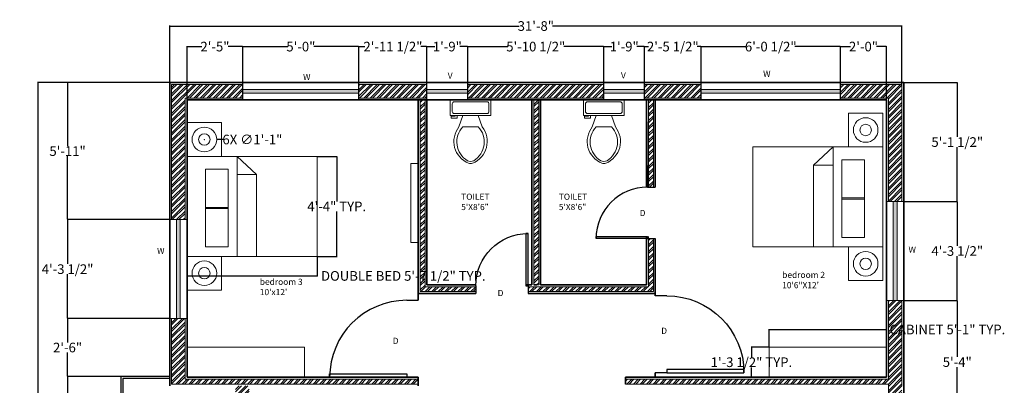
# Model space of a CAD drawing. Units: inches. Extents: x -340 to 394, y 381 to 1380.
# Tile 3 of 3: x -117 to 394, y 757 to 947. Entities that reach past the tile are written whole.
import ezdxf

# ---------------------------------------------------------------- set-up
doc = ezdxf.new("R2010")
doc.units = ezdxf.units.IN
doc.header["$MEASUREMENT"] = 0
for name, color, linetype, lineweight in [('A-ANNO-DIMS', 150, 'Continuous', 18), ('A-ANNO-TEXT', 11, 'Continuous', 18), ('A-AREA-IDEN', 11, 'Continuous', 18), ('A-FLOR', 150, 'Continuous', 25), ('A-FLOR-CASE', 130, 'Continuous', 20), ('A-FLOR-FIXT', 130, 'Continuous', 18), ('A-GLAZ-PATT', 220, 'Continuous', 13), ('A-WALL-FNSH', 150, 'Continuous', 18), ('A-WALL-PATT', 10, 'Continuous', 13), ('door', 200, 'Continuous', 25), ('fur', 130, 'Continuous', 18), ('wall', 150, 'Continuous', 35), ('wind', 220, 'Continuous', 20)]:
    doc.layers.add(name, color=color, linetype=linetype, lineweight=lineweight)
doc.styles.get("Standard").update_dxf_attribs({"font": 'arial.ttf'})
doc.dimstyles.get("Standard").update_dxf_attribs({"dimtxt": 5, "dimasz": 0.18, "dimexe": 0.18, "dimexo": 0.0625, "dimgap": 0.09, "dimtad": 0, "dimtih": 1, "dimtoh": 1, "dimdec": 0, "dimzin": 0, "dimdsep": 46, "dimlunit": 4, "dimtxsty": 'Standard', "dimcen": 0.09, "dimadec": 0, "dimazin": 0, "dimtfac": 1, "dimtdec": 0, "dimtofl": 0, "dimtmove": 0, "dimatfit": 3, "dimfxl": 1, "dimtolj": 1, "dimtzin": 0, "dimarcsym": 0})

# ---------------------------------------------------------------- blocks, each defined once
blk = doc.blocks.new('*U2')
for p, q in [((0, 0), (0, -6)), ((40, 0), (40, -6))]:
    blk.add_line(p, q)
blk.add_lwpolyline([(0, 0), (0, 40), (1.75, 40), (1.75, 0)], close=True)
blk.add_arc((0, 0), 40, 0, 90)
blk = doc.blocks.new('*U4')
for p, q in [((9.5, -6), (9.5, -2)), ((-10, -8.5), (-8, -8.5)), ((-10, -9.5), (-10, -8.5)), ((-7, -9.5), (-10, -9.5)), ((-8, -8.5), (-8, -8)), ((-7, -8), (-7, -9.5)), ((-4, -8), (-6, -14)), ((4, -8), (6, -14)), ((4, -14), (-4, -14))]:
    blk.add_line(p, q)
blk.add_lwpolyline([(10.5, -8), (10.5, 0), (-10.5, 0), (-10.5, -8)], close=True)
for points in [[(-9.5, -2), (-9.5, -6)], [(8.5, -1), (-8.5, -1)], [(-8.5, -7), (8.5, -7)]]:
    blk.add_lwpolyline(points)
for centre, radius, start, end in [((-8.62, -1.88), 0.884, 81.8699, 188.1301), ((8.62, -1.88), 0.884, 351.8699, 98.1301), ((-8.62, -6.12), 0.884, 171.8699, 278.1301), ((8.62, -6.12), 0.884, 261.8699, 8.1301), ((3.52, -21.58), 12.17, 141.4691, 247.9714), ((4.2, -21.82), 11.33, 136.3677, 238.9468), ((-3.52, -21.58), 12.17, 292.0284, 38.5307), ((-4.2, -21.82), 11.33, 301.053, 43.6321), ((0, -27.88), 4, 245.7318, 294.2682), ((0, -29), 4, 254.8605, 285.1395)]:
    blk.add_arc(centre, radius, start, end)
blk = doc.blocks.new('*D5')
at = {"layer": 'A-ANNO-DIMS', "color": 0, "lineweight": -2, "transparency": 16777216}
for p, q in [((-39.62, 914.26), (-39.62, 943.76)), ((-39.44, 943.58), (141.71, 943.58)), ((340.2, 943.58), (159.06, 943.58)), ((340.38, 913.26), (340.38, 943.76))]:
    blk.add_line(p, q, dxfattribs=at)
at = {"layer": 'A-ANNO-DIMS', "color": 0, "transparency": 16777216}
for points in [[(-39.44, 943.61), (-39.44, 943.55), (-39.62, 943.58)], [(340.2, 943.61), (340.2, 943.55), (340.38, 943.58)]]:
    blk.add_solid(points, dxfattribs=at)
at = {"layer": 'Defpoints', "color": 0, "transparency": 16777216}
for p in [(340.38, 943.58), (-39.62, 914.2), (340.38, 913.2)]:
    blk.add_point(p, dxfattribs=at)
at = {"layer": 'A-ANNO-DIMS', "color": 0, "transparency": 16777216, "insert": (150.38, 943.58), "char_height": 5, "attachment_point": 5}
blk.add_mtext('\\A1;31\'-8"', dxfattribs=at)
blk = doc.blocks.new('*D6')
at = {"layer": 'A-ANNO-DIMS', "color": 0, "lineweight": -2, "transparency": 16777216}
for p, q in [((-39.68, 914.2), (-108.24, 914.2)), ((-108.06, 914.02), (-108.06, 693.34)), ((-108.06, 467.38), (-108.06, 688.05)), ((-39.68, 467.2), (-108.24, 467.2))]:
    blk.add_line(p, q, dxfattribs=at)
at = {"layer": 'A-ANNO-DIMS', "color": 0, "transparency": 16777216}
for points in [[(-108.09, 914.02), (-108.03, 914.02), (-108.06, 914.2)], [(-108.09, 467.38), (-108.03, 467.38), (-108.06, 467.2)]]:
    blk.add_solid(points, dxfattribs=at)
at = {"layer": 'Defpoints', "color": 0, "transparency": 16777216}
for p in [(-39.62, 914.2), (-108.06, 467.2), (-39.62, 467.2)]:
    blk.add_point(p, dxfattribs=at)
at = {"layer": 'A-ANNO-DIMS', "color": 0, "transparency": 16777216, "insert": (-108.06, 690.7), "char_height": 5, "attachment_point": 5}
blk.add_mtext('\\A1;37\'-3"', dxfattribs=at)
blk = doc.blocks.new('BED-DOUBLE')
for p, q in [((25.93, 0), (25.93, 51.94)), ((25.93, 51.94), (25.93, 42.46)), ((36.06, 42.46), (25.93, 51.94)), ((25.93, 51.94), (36.06, 42.46)), ((25.93, 42.46), (36.06, 42.46)), ((36.06, 42.46), (36.06, 0))]:
    blk.add_line(p, q)
for points in [[(0, 0), (67.52, 0), (67.52, 51.94), (0, 51.94)], [(9.57, 24.81), (21.34, 24.81), (21.34, 45.28), (9.57, 45.28)], [(9.57, 4.93), (21.34, 4.93), (21.34, 25.4), (9.57, 25.4)]]:
    blk.add_lwpolyline(points, close=True)
blk = doc.blocks.new('NIGHTSTAND')
blk.add_lwpolyline([(0, 0), (17.94, 0), (17.94, 17.5), (0, 17.5)], close=True)
for radius in [6.39, 2.96]:
    blk.add_circle((8.97, 8.75), radius)
blk = doc.blocks.new('CABINET-BEDROOM')
blk.add_lwpolyline([(0, 0), (60.98, 0), (60.98, 15.69), (0, 15.69)], close=True)
blk = doc.blocks.new('*D15')
at = {"layer": 'A-ANNO-DIMS', "color": 0, "lineweight": -2, "transparency": 16777216}
for p, q in [((-30.62, 823.92), (-30.62, 813.67)), ((36.9, 823.92), (36.9, 813.67)), ((-30.44, 813.85), (36.72, 813.85)), ((36.9, 813.85), (37.08, 813.85))]:
    blk.add_line(p, q, dxfattribs=at)
at = {"layer": 'A-ANNO-DIMS', "color": 0, "transparency": 16777216}
for points in [[(-30.44, 813.88), (-30.44, 813.82), (-30.62, 813.85)], [(36.72, 813.88), (36.72, 813.82), (36.9, 813.85)]]:
    blk.add_solid(points, dxfattribs=at)
at = {"layer": 'Defpoints', "color": 0, "transparency": 16777216}
for p in [(-30.62, 823.98), (36.9, 823.98), (36.9, 813.85)]:
    blk.add_point(p, dxfattribs=at)
at = {"layer": 'A-ANNO-DIMS', "color": 0, "transparency": 16777216, "insert": (81.59, 813.85), "char_height": 5, "attachment_point": 5}
blk.add_mtext('\\A1;DOUBLE BED 5\'-7 1/2" TYP.', dxfattribs=at)
blk = doc.blocks.new('*D16')
at = {"layer": 'A-ANNO-DIMS', "color": 0, "lineweight": -2, "transparency": 16777216}
for p, q in [((36.96, 875.92), (47.21, 875.92)), ((47.03, 875.74), (47.03, 852.54)), ((47.03, 824.16), (47.03, 847.36)), ((36.96, 823.98), (47.21, 823.98))]:
    blk.add_line(p, q, dxfattribs=at)
at = {"layer": 'A-ANNO-DIMS', "color": 0, "transparency": 16777216}
for points in [[(47, 875.74), (47.06, 875.74), (47.03, 875.92)], [(47, 824.16), (47.06, 824.16), (47.03, 823.98)]]:
    blk.add_solid(points, dxfattribs=at)
at = {"layer": 'Defpoints', "color": 0, "transparency": 16777216}
for p in [(36.9, 875.92), (47.03, 875.92), (36.9, 823.98)]:
    blk.add_point(p, dxfattribs=at)
at = {"layer": 'A-ANNO-DIMS', "color": 0, "transparency": 16777216, "insert": (47.03, 849.95), "char_height": 5, "attachment_point": 5}
blk.add_mtext('\\A1;4\'-4" TYP.', dxfattribs=at)
blk = doc.blocks.new('*D17')
at = {"layer": 'A-ANNO-DIMS', "color": 0, "lineweight": -2, "transparency": 16777216}
for p, q in [((271.4, 776.95), (271.4, 786.21)), ((271.58, 786.03), (332.2, 786.03)), ((332.38, 776.95), (332.38, 786.21)), ((332.38, 786.03), (332.56, 786.03))]:
    blk.add_line(p, q, dxfattribs=at)
at = {"layer": 'A-ANNO-DIMS', "color": 0, "transparency": 16777216}
for points in [[(271.58, 786.06), (271.58, 786), (271.4, 786.03)], [(332.2, 786.06), (332.2, 786), (332.38, 786.03)]]:
    blk.add_solid(points, dxfattribs=at)
at = {"layer": 'Defpoints', "color": 0, "transparency": 16777216}
for p in [(332.38, 786.03), (271.4, 776.89), (332.38, 776.89)]:
    blk.add_point(p, dxfattribs=at)
at = {"layer": 'A-ANNO-DIMS', "color": 0, "transparency": 16777216, "insert": (363.97, 786.03), "char_height": 5, "attachment_point": 5}
blk.add_mtext('\\A1;CABINET 5\'-1" TYP.', dxfattribs=at)
blk = doc.blocks.new('*D18')
at = {"layer": 'A-ANNO-DIMS', "color": 0, "lineweight": -2, "transparency": 16777216}
for p, q in [((271.34, 776.89), (262.08, 776.89)), ((262.26, 776.71), (262.26, 771.72)), ((262.26, 761.38), (262.26, 766.37)), ((271.34, 761.2), (262.08, 761.2))]:
    blk.add_line(p, q, dxfattribs=at)
at = {"layer": 'A-ANNO-DIMS', "color": 0, "transparency": 16777216}
for points in [[(262.23, 776.71), (262.29, 776.71), (262.26, 776.89)], [(262.23, 761.38), (262.29, 761.38), (262.26, 761.2)]]:
    blk.add_solid(points, dxfattribs=at)
at = {"layer": 'Defpoints', "color": 0, "transparency": 16777216}
for p in [(262.26, 776.89), (271.4, 776.89), (271.4, 761.2)]:
    blk.add_point(p, dxfattribs=at)
at = {"layer": 'A-ANNO-DIMS', "color": 0, "transparency": 16777216, "insert": (262.26, 769.04), "char_height": 5, "attachment_point": 5}
blk.add_mtext('\\A1;1\'-3 1/2" TYP.', dxfattribs=at)
blk = doc.blocks.new('*D29')
at = {"layer": 'A-ANNO-DIMS', "color": 0, "lineweight": -2, "transparency": 16777216}
for p, q in [((341.44, 801.11), (369.26, 801.11)), ((369.08, 800.93), (369.08, 771.76)), ((369.08, 737.33), (369.08, 766.49)), ((341.44, 737.15), (369.26, 737.15))]:
    blk.add_line(p, q, dxfattribs=at)
at = {"layer": 'A-ANNO-DIMS', "color": 0, "transparency": 16777216}
for points in [[(369.05, 800.93), (369.11, 800.93), (369.08, 801.11)], [(369.05, 737.33), (369.11, 737.33), (369.08, 737.15)]]:
    blk.add_solid(points, dxfattribs=at)
at = {"layer": 'Defpoints', "color": 0, "transparency": 16777216}
for p in [(341.38, 801.11), (369.08, 801.11), (341.38, 737.15)]:
    blk.add_point(p, dxfattribs=at)
at = {"layer": 'A-ANNO-DIMS', "color": 0, "transparency": 16777216, "insert": (369.08, 769.13), "char_height": 5, "attachment_point": 5}
blk.add_mtext('\\A1;5\'-4"', dxfattribs=at)
blk = doc.blocks.new('*D30')
at = {"layer": 'A-ANNO-DIMS', "color": 0, "lineweight": -2, "transparency": 16777216}
for p, q in [((341.44, 852.47), (369.26, 852.47)), ((369.08, 852.29), (369.08, 829.47)), ((369.08, 801.29), (369.08, 824.11)), ((341.44, 801.11), (369.26, 801.11))]:
    blk.add_line(p, q, dxfattribs=at)
at = {"layer": 'A-ANNO-DIMS', "color": 0, "transparency": 16777216}
for points in [[(369.05, 852.29), (369.11, 852.29), (369.08, 852.47)], [(369.05, 801.29), (369.11, 801.29), (369.08, 801.11)]]:
    blk.add_solid(points, dxfattribs=at)
at = {"layer": 'Defpoints', "color": 0, "transparency": 16777216}
for p in [(341.38, 852.47), (369.08, 852.47), (341.38, 801.11)]:
    blk.add_point(p, dxfattribs=at)
at = {"layer": 'A-ANNO-DIMS', "color": 0, "transparency": 16777216, "insert": (369.08, 826.79), "char_height": 5, "attachment_point": 5}
blk.add_mtext('\\A1;4\'-3 1/2"', dxfattribs=at)
blk = doc.blocks.new('*D31')
at = {"layer": 'A-ANNO-DIMS', "color": 0, "lineweight": -2, "transparency": 16777216}
for p, q in [((341.44, 914.2), (369.26, 914.2)), ((369.08, 914.02), (369.08, 886.01)), ((369.08, 852.65), (369.08, 880.66)), ((341.44, 852.47), (369.26, 852.47))]:
    blk.add_line(p, q, dxfattribs=at)
at = {"layer": 'A-ANNO-DIMS', "color": 0, "transparency": 16777216}
for points in [[(369.05, 914.02), (369.11, 914.02), (369.08, 914.2)], [(369.05, 852.65), (369.11, 852.65), (369.08, 852.47)]]:
    blk.add_solid(points, dxfattribs=at)
at = {"layer": 'Defpoints', "color": 0, "transparency": 16777216}
for p in [(341.38, 914.2), (369.08, 914.2), (341.38, 852.47)]:
    blk.add_point(p, dxfattribs=at)
at = {"layer": 'A-ANNO-DIMS', "color": 0, "transparency": 16777216, "insert": (369.08, 883.34), "char_height": 5, "attachment_point": 5}
blk.add_mtext('\\A1;5\'-1 1/2"', dxfattribs=at)
blk = doc.blocks.new('*D32')
at = {"layer": 'A-ANNO-DIMS', "color": 0, "lineweight": -2, "transparency": 16777216}
for p, q in [((-30.62, 905.26), (-30.62, 933.08)), ((-30.44, 932.9), (-22.93, 932.9)), ((-1.86, 932.9), (-9.37, 932.9)), ((-1.68, 905.26), (-1.68, 933.08))]:
    blk.add_line(p, q, dxfattribs=at)
at = {"layer": 'A-ANNO-DIMS', "color": 0, "transparency": 16777216}
for points in [[(-30.44, 932.93), (-30.44, 932.87), (-30.62, 932.9)], [(-1.86, 932.93), (-1.86, 932.87), (-1.68, 932.9)]]:
    blk.add_solid(points, dxfattribs=at)
at = {"layer": 'Defpoints', "color": 0, "transparency": 16777216}
for p in [(-1.68, 932.9), (-30.62, 905.2), (-1.68, 905.2)]:
    blk.add_point(p, dxfattribs=at)
at = {"layer": 'A-ANNO-DIMS', "color": 0, "transparency": 16777216, "insert": (-16.15, 932.9), "char_height": 5, "attachment_point": 5}
blk.add_mtext('\\A1;2\'-5"', dxfattribs=at)
blk = doc.blocks.new('*D33')
at = {"layer": 'A-ANNO-DIMS', "color": 0, "lineweight": -2, "transparency": 16777216}
for p, q in [((-1.68, 905.26), (-1.68, 933.08)), ((-1.5, 932.9), (21.71, 932.9)), ((58.38, 932.9), (35.18, 932.9)), ((58.56, 905.26), (58.56, 933.08))]:
    blk.add_line(p, q, dxfattribs=at)
at = {"layer": 'A-ANNO-DIMS', "color": 0, "transparency": 16777216}
for points in [[(-1.5, 932.93), (-1.5, 932.87), (-1.68, 932.9)], [(58.38, 932.93), (58.38, 932.87), (58.56, 932.9)]]:
    blk.add_solid(points, dxfattribs=at)
at = {"layer": 'Defpoints', "color": 0, "transparency": 16777216}
for p in [(58.56, 932.9), (-1.68, 905.2), (58.56, 905.2)]:
    blk.add_point(p, dxfattribs=at)
at = {"layer": 'A-ANNO-DIMS', "color": 0, "transparency": 16777216, "insert": (28.44, 932.9), "char_height": 5, "attachment_point": 5}
blk.add_mtext('\\A1;5\'-0"', dxfattribs=at)
blk = doc.blocks.new('*D34')
at = {"layer": 'A-ANNO-DIMS', "color": 0, "lineweight": -2, "transparency": 16777216}
for p, q in [((58.56, 905.26), (58.56, 933.08)), ((58.74, 932.9), (61.68, 932.9)), ((93.7, 932.9), (90.77, 932.9)), ((93.88, 905.26), (93.88, 933.08))]:
    blk.add_line(p, q, dxfattribs=at)
at = {"layer": 'A-ANNO-DIMS', "color": 0, "transparency": 16777216}
for points in [[(58.74, 932.93), (58.74, 932.87), (58.56, 932.9)], [(93.7, 932.93), (93.7, 932.87), (93.88, 932.9)]]:
    blk.add_solid(points, dxfattribs=at)
at = {"layer": 'Defpoints', "color": 0, "transparency": 16777216}
for p in [(93.88, 932.9), (58.56, 905.2), (93.88, 905.2)]:
    blk.add_point(p, dxfattribs=at)
at = {"layer": 'A-ANNO-DIMS', "color": 0, "transparency": 16777216, "insert": (76.22, 932.9), "char_height": 5, "attachment_point": 5}
blk.add_mtext('\\A1;2\'-11 1/2"', dxfattribs=at)
blk = doc.blocks.new('*D35')
at = {"layer": 'A-ANNO-DIMS', "color": 0, "lineweight": -2, "transparency": 16777216}
for p, q in [((93.88, 905.26), (93.88, 933.08)), ((94.06, 932.9), (97.95, 932.9)), ((114.84, 932.9), (110.95, 932.9)), ((115.02, 905.26), (115.02, 933.08))]:
    blk.add_line(p, q, dxfattribs=at)
at = {"layer": 'A-ANNO-DIMS', "color": 0, "transparency": 16777216}
for points in [[(94.06, 932.93), (94.06, 932.87), (93.88, 932.9)], [(114.84, 932.93), (114.84, 932.87), (115.02, 932.9)]]:
    blk.add_solid(points, dxfattribs=at)
at = {"layer": 'Defpoints', "color": 0, "transparency": 16777216}
for p in [(115.02, 932.9), (93.88, 905.2), (115.02, 905.2)]:
    blk.add_point(p, dxfattribs=at)
at = {"layer": 'A-ANNO-DIMS', "color": 0, "transparency": 16777216, "insert": (104.45, 932.9), "char_height": 5, "attachment_point": 5}
blk.add_mtext('\\A1;1\'-9"', dxfattribs=at)
blk = doc.blocks.new('*D36')
at = {"layer": 'A-ANNO-DIMS', "color": 0, "lineweight": -2, "transparency": 16777216}
for p, q in [((115.02, 905.26), (115.02, 933.08)), ((115.2, 932.9), (135.84, 932.9)), ((185.49, 932.9), (164.85, 932.9)), ((185.67, 905.26), (185.67, 933.08))]:
    blk.add_line(p, q, dxfattribs=at)
at = {"layer": 'A-ANNO-DIMS', "color": 0, "transparency": 16777216}
for points in [[(115.2, 932.93), (115.2, 932.87), (115.02, 932.9)], [(185.49, 932.93), (185.49, 932.87), (185.67, 932.9)]]:
    blk.add_solid(points, dxfattribs=at)
at = {"layer": 'Defpoints', "color": 0, "transparency": 16777216}
for p in [(185.67, 932.9), (115.02, 905.2), (185.67, 905.2)]:
    blk.add_point(p, dxfattribs=at)
at = {"layer": 'A-ANNO-DIMS', "color": 0, "transparency": 16777216, "insert": (150.34, 932.9), "char_height": 5, "attachment_point": 5}
blk.add_mtext('\\A1;5\'-10 1/2"', dxfattribs=at)
blk = doc.blocks.new('*D37')
at = {"layer": 'A-ANNO-DIMS', "color": 0, "lineweight": -2, "transparency": 16777216}
for p, q in [((185.67, 905.26), (185.67, 933.08)), ((185.85, 932.9), (189.74, 932.9)), ((206.62, 932.9), (202.74, 932.9)), ((206.8, 905.26), (206.8, 933.08))]:
    blk.add_line(p, q, dxfattribs=at)
at = {"layer": 'A-ANNO-DIMS', "color": 0, "transparency": 16777216}
for points in [[(185.85, 932.93), (185.85, 932.87), (185.67, 932.9)], [(206.62, 932.93), (206.62, 932.87), (206.8, 932.9)]]:
    blk.add_solid(points, dxfattribs=at)
at = {"layer": 'Defpoints', "color": 0, "transparency": 16777216}
for p in [(206.8, 932.9), (185.67, 905.2), (206.8, 905.2)]:
    blk.add_point(p, dxfattribs=at)
at = {"layer": 'A-ANNO-DIMS', "color": 0, "transparency": 16777216, "insert": (196.24, 932.9), "char_height": 5, "attachment_point": 5}
blk.add_mtext('\\A1;1\'-9"', dxfattribs=at)
blk = doc.blocks.new('*D38')
at = {"layer": 'A-ANNO-DIMS', "color": 0, "lineweight": -2, "transparency": 16777216}
for p, q in [((206.8, 905.26), (206.8, 933.08)), ((206.98, 932.9), (208.86, 932.9)), ((235.94, 932.9), (234.06, 932.9)), ((236.12, 905.26), (236.12, 933.08))]:
    blk.add_line(p, q, dxfattribs=at)
at = {"layer": 'A-ANNO-DIMS', "color": 0, "transparency": 16777216}
for points in [[(206.98, 932.93), (206.98, 932.87), (206.8, 932.9)], [(235.94, 932.93), (235.94, 932.87), (236.12, 932.9)]]:
    blk.add_solid(points, dxfattribs=at)
at = {"layer": 'Defpoints', "color": 0, "transparency": 16777216}
for p in [(236.12, 932.9), (206.8, 905.2), (236.12, 905.2)]:
    blk.add_point(p, dxfattribs=at)
at = {"layer": 'A-ANNO-DIMS', "color": 0, "transparency": 16777216, "insert": (221.46, 932.9), "char_height": 5, "attachment_point": 5}
blk.add_mtext('\\A1;2\'-5 1/2"', dxfattribs=at)
blk = doc.blocks.new('*D39')
at = {"layer": 'A-ANNO-DIMS', "color": 0, "lineweight": -2, "transparency": 16777216}
for p, q in [((236.12, 905.26), (236.12, 933.08)), ((236.3, 932.9), (259.72, 932.9)), ((308.3, 932.9), (284.87, 932.9)), ((308.48, 905.26), (308.48, 933.08))]:
    blk.add_line(p, q, dxfattribs=at)
at = {"layer": 'A-ANNO-DIMS', "color": 0, "transparency": 16777216}
for points in [[(236.3, 932.93), (236.3, 932.87), (236.12, 932.9)], [(308.3, 932.93), (308.3, 932.87), (308.48, 932.9)]]:
    blk.add_solid(points, dxfattribs=at)
at = {"layer": 'Defpoints', "color": 0, "transparency": 16777216}
for p in [(308.48, 932.9), (236.12, 905.2), (308.48, 905.2)]:
    blk.add_point(p, dxfattribs=at)
at = {"layer": 'A-ANNO-DIMS', "color": 0, "transparency": 16777216, "insert": (272.3, 932.9), "char_height": 5, "attachment_point": 5}
blk.add_mtext('\\A1;6\'-0 1/2"', dxfattribs=at)
blk = doc.blocks.new('*D40')
at = {"layer": 'A-ANNO-DIMS', "color": 0, "lineweight": -2, "transparency": 16777216}
for p, q in [((308.48, 905.26), (308.48, 933.08)), ((308.66, 932.9), (313.65, 932.9)), ((332.2, 932.9), (327.21, 932.9)), ((332.38, 905.26), (332.38, 933.08))]:
    blk.add_line(p, q, dxfattribs=at)
at = {"layer": 'A-ANNO-DIMS', "color": 0, "transparency": 16777216}
for points in [[(308.66, 932.93), (308.66, 932.87), (308.48, 932.9)], [(332.2, 932.93), (332.2, 932.87), (332.38, 932.9)]]:
    blk.add_solid(points, dxfattribs=at)
at = {"layer": 'Defpoints', "color": 0, "transparency": 16777216}
for p in [(332.38, 932.9), (308.48, 905.2), (332.38, 905.2)]:
    blk.add_point(p, dxfattribs=at)
at = {"layer": 'A-ANNO-DIMS', "color": 0, "transparency": 16777216, "insert": (320.43, 932.9), "char_height": 5, "attachment_point": 5}
blk.add_mtext('\\A1;2\'-0"', dxfattribs=at)
blk = doc.blocks.new('*D42')
at = {"layer": 'A-ANNO-DIMS', "color": 0, "lineweight": -2, "transparency": 16777216}
for p, q in [((-65, 761.64), (-92.82, 761.64)), ((-92.64, 761.46), (-92.64, 693.71)), ((-92.64, 620.68), (-92.64, 688.43)), ((-65, 620.5), (-92.82, 620.5))]:
    blk.add_line(p, q, dxfattribs=at)
at = {"layer": 'A-ANNO-DIMS', "color": 0, "transparency": 16777216}
for points in [[(-92.67, 761.46), (-92.61, 761.46), (-92.64, 761.64)], [(-92.67, 620.68), (-92.61, 620.68), (-92.64, 620.5)]]:
    blk.add_solid(points, dxfattribs=at)
at = {"layer": 'Defpoints', "color": 0, "transparency": 16777216}
for p in [(-92.64, 761.64), (-64.94, 761.64), (-64.94, 620.5)]:
    blk.add_point(p, dxfattribs=at)
at = {"layer": 'A-ANNO-DIMS', "color": 0, "transparency": 16777216, "insert": (-92.64, 691.07), "char_height": 5, "attachment_point": 5}
blk.add_mtext('\\A1;11\'-9"', dxfattribs=at)
blk = doc.blocks.new('*D43')
at = {"layer": 'A-ANNO-DIMS', "color": 0, "lineweight": -2, "transparency": 16777216}
for p, q in [((-39.68, 791.69), (-92.82, 791.69)), ((-92.64, 791.51), (-92.64, 779.31)), ((-92.64, 761.82), (-92.64, 774.02)), ((-65, 761.64), (-92.82, 761.64))]:
    blk.add_line(p, q, dxfattribs=at)
at = {"layer": 'A-ANNO-DIMS', "color": 0, "transparency": 16777216}
for points in [[(-92.67, 791.51), (-92.61, 791.51), (-92.64, 791.69)], [(-92.67, 761.82), (-92.61, 761.82), (-92.64, 761.64)]]:
    blk.add_solid(points, dxfattribs=at)
at = {"layer": 'Defpoints', "color": 0, "transparency": 16777216}
for p in [(-92.64, 791.69), (-39.62, 791.69), (-64.94, 761.64)]:
    blk.add_point(p, dxfattribs=at)
at = {"layer": 'A-ANNO-DIMS', "color": 0, "transparency": 16777216, "insert": (-92.64, 776.67), "char_height": 5, "attachment_point": 5}
blk.add_mtext('\\A1;2\'-6"', dxfattribs=at)
blk = doc.blocks.new('*D44')
at = {"layer": 'A-ANNO-DIMS', "color": 0, "lineweight": -2, "transparency": 16777216}
for p, q in [((-39.68, 843.05), (-92.82, 843.05)), ((-92.64, 842.87), (-92.64, 820.05)), ((-92.64, 791.87), (-92.64, 814.69)), ((-39.68, 791.69), (-92.82, 791.69))]:
    blk.add_line(p, q, dxfattribs=at)
at = {"layer": 'A-ANNO-DIMS', "color": 0, "transparency": 16777216}
for points in [[(-92.67, 842.87), (-92.61, 842.87), (-92.64, 843.05)], [(-92.67, 791.87), (-92.61, 791.87), (-92.64, 791.69)]]:
    blk.add_solid(points, dxfattribs=at)
at = {"layer": 'Defpoints', "color": 0, "transparency": 16777216}
for p in [(-92.64, 843.05), (-39.62, 843.05), (-39.62, 791.69)]:
    blk.add_point(p, dxfattribs=at)
at = {"layer": 'A-ANNO-DIMS', "color": 0, "transparency": 16777216, "insert": (-92.64, 817.37), "char_height": 5, "attachment_point": 5}
blk.add_mtext('\\A1;4\'-3 1/2"', dxfattribs=at)
blk = doc.blocks.new('*D45')
at = {"layer": 'A-ANNO-DIMS', "color": 0, "lineweight": -2, "transparency": 16777216}
for p, q in [((-39.68, 914.2), (-92.82, 914.2)), ((-92.64, 914.02), (-92.64, 881.27)), ((-92.64, 843.23), (-92.64, 875.98)), ((-39.68, 843.05), (-92.82, 843.05))]:
    blk.add_line(p, q, dxfattribs=at)
at = {"layer": 'A-ANNO-DIMS', "color": 0, "transparency": 16777216}
for points in [[(-92.67, 914.02), (-92.61, 914.02), (-92.64, 914.2)], [(-92.67, 843.23), (-92.61, 843.23), (-92.64, 843.05)]]:
    blk.add_solid(points, dxfattribs=at)
at = {"layer": 'Defpoints', "color": 0, "transparency": 16777216}
for p in [(-92.64, 914.2), (-39.62, 914.2), (-39.62, 843.05)]:
    blk.add_point(p, dxfattribs=at)
at = {"layer": 'A-ANNO-DIMS', "color": 0, "transparency": 16777216, "insert": (-92.64, 878.63), "char_height": 5, "attachment_point": 5}
blk.add_mtext('\\A1;5\'-11"', dxfattribs=at)
blk = doc.blocks.new('*D60')
at = {"layer": 'A-ANNO-DIMS', "color": 0, "lineweight": -2, "transparency": 16777216}
for p, q in [((-21.74, 884.67), (-21.56, 884.67)), ((-21.65, 884.58), (-21.65, 884.76)), ((-11.43, 884.67), (-15.08, 884.67))]:
    blk.add_line(p, q, dxfattribs=at)
at = {"layer": 'A-ANNO-DIMS', "color": 0, "transparency": 16777216}
blk.add_solid([(-15.08, 884.7), (-15.08, 884.64), (-15.26, 884.67)], dxfattribs=at)
at = {"layer": 'Defpoints', "color": 0, "transparency": 16777216}
for p in [(-28.04, 884.67), (-15.26, 884.67)]:
    blk.add_point(p, dxfattribs=at)
at = {"layer": 'A-ANNO-DIMS', "color": 0, "transparency": 16777216, "insert": (3.28, 884.67), "char_height": 5, "attachment_point": 5}
blk.add_mtext('\\A1;6X ∅1\'-1"', dxfattribs=at)

msp = doc.modelspace()

# ---------------------------------------------------------------- hatches: boundary and pattern name
at = {"layer": 'A-GLAZ-PATT'}
h = msp.add_hatch(color=256, dxfattribs=at)
h.dxf.hatch_style = 1
h.paths.add_polyline_path([(58.56, 910.7), (-1.68, 910.7), (-1.68, 908.7), (58.56, 908.7)])
h.paths.add_polyline_path([(115.02, 910.7), (93.88, 910.7), (93.88, 908.7), (115.02, 908.7)])
h.paths.add_polyline_path([(206.8, 910.7), (185.67, 910.7), (185.67, 908.7), (206.8, 908.7)])
h.paths.add_polyline_path([(308.48, 910.7), (236.12, 910.7), (236.12, 908.7), (308.48, 908.7)])
h.paths.add_polyline_path([(337.88, 852.47), (335.88, 852.47), (335.88, 801.11), (337.88, 801.11)])
h.paths.add_polyline_path([(-34.12, 843.05), (-36.12, 843.05), (-36.12, 791.69), (-34.12, 791.69)])
h.paths.add_polyline_path([(-0.92, 737.98), (-2.92, 737.98), (-2.92, 646.31), (-0.92, 646.31)])
h.paths.add_polyline_path([(337.88, 685.13), (335.88, 685.13), (335.88, 633.76), (337.88, 633.76)])
h.paths.add_polyline_path([(19, 527.45), (-19.67, 527.45), (-19.67, 525.45), (19, 525.45)])
h.paths.add_polyline_path([(63.15, 472.7), (2.91, 472.7), (2.91, 470.7), (63.15, 470.7)])
h.paths.add_polyline_path([(121.02, 472.7), (99.88, 472.7), (99.88, 470.7), (121.02, 470.7)])
h.paths.add_polyline_path([(310.81, 472.7), (272.96, 472.7), (272.96, 470.7), (310.81, 470.7)])
h.paths.add_polyline_path([(209.39, 472.7), (171.54, 472.7), (171.54, 470.7), (209.39, 470.7)])
at = {"layer": 'A-WALL-PATT'}
h = msp.add_hatch(dxfattribs=at)
h.set_pattern_fill('ANSI32', color=256, scale=6.4)
h.paths.add_polyline_path([(-31.62, 906.2), (-1.68, 906.2), (-1.68, 913.2), (-38.62, 913.2), (-38.62, 843.05), (-31.62, 843.05)])
h.paths.add_polyline_path([(93.88, 913.2), (58.56, 913.2), (58.56, 906.2), (93.88, 906.2)])
h.paths.add_polyline_path([(185.67, 913.2), (141.88, 913.2), (115.02, 913.2), (115.02, 906.2), (185.67, 906.2)])
h.paths.add_polyline_path([(151.88, 905.2), (149.38, 905.2), (149.38, 809.2), (151.88, 809.2)])
h.paths.add_polyline_path([(236.12, 913.2), (206.8, 913.2), (206.8, 906.2), (207.88, 906.2), (236.12, 906.2)])
h.paths.add_polyline_path([(340.38, 913.2), (308.48, 913.2), (308.48, 906.2), (333.38, 906.2), (333.38, 852.47), (340.38, 852.47)])
h = msp.add_hatch(dxfattribs=at)
h.set_pattern_fill('ANSI32', color=256, scale=6.4)
h.paths.add_polyline_path([(211.38, 905.2), (208.88, 905.2), (208.88, 859.96), (211.38, 859.96)])
h.paths.add_polyline_path([(211.38, 833.2), (208.88, 833.2), (208.88, 808.2), (146.36, 808.2), (146.36, 805.7), (211.38, 805.7)])
h.paths.add_polyline_path([(92.88, 905.2), (90.38, 905.2), (90.38, 805.7), (119.27, 805.7), (119.27, 808.2), (92.88, 808.2)])
h.paths.add_polyline_path([(1.58, 756.7), (-5.42, 756.7), (-5.42, 737.98), (1.58, 737.98)], flags=17)
h.paths.add_polyline_path([(1.58, 646.31), (-5.42, 646.31), (-5.42, 629.2), (1.58, 629.2)])
h.paths.add_polyline_path([(340.38, 697.15), (335.38, 697.15, -0.012506), (333.38, 697.2), (333.38, 685.13), (340.38, 685.13)])
h.paths.add_polyline_path([(29.76, 527.7), (19, 527.7), (19, 525.2), (29.76, 525.2)], flags=17)
h.paths.add_polyline_path([(98.88, 579.2), (160.88, 579.2), (160.88, 548.2), (161.03, 548.2), (163.38, 548.2), (163.38, 621.2), (165.94, 621.2), (165.94, 623.7), (160.88, 623.7), (160.88, 581.7), (96.38, 581.7), (96.38, 527.7), (69.71, 527.7), (69.71, 525.2), (96.38, 525.2), (96.38, 475.2), (63.15, 475.2), (63.15, 468.2), (98.88, 468.2)])
h.paths.add_polyline_path([(171.54, 475.2), (163.38, 475.2), (163.38, 525.87), (160.88, 525.87), (160.88, 475.2), (121.02, 475.2), (121.02, 468.2), (159.88, 468.2), (171.54, 468.2)])
h.paths.add_polyline_path([(272.96, 475.2), (209.39, 475.2), (209.39, 468.2), (272.96, 468.2)], flags=17)
h.paths.add_polyline_path([(340.38, 620.2), (340.38, 633.76), (333.38, 633.76), (333.38, 623.7), (205.94, 623.7), (205.94, 621.2), (333.38, 621.2), (333.38, 475.2), (310.81, 475.2), (310.81, 468.2), (340.38, 468.2)])
h = msp.add_hatch(dxfattribs=at)
h.set_pattern_fill('ANSI32', color=256, scale=6.4)
h.paths.add_polyline_path([(116.88, 628.2), (-38.62, 628.2), (-38.62, 528.7), (-38.62, 468.2), (2.91, 468.2), (2.91, 475.2), (-31.62, 475.2), (-31.62, 525.2), (-19.67, 525.2), (-19.67, 527.7), (-31.62, 527.7), (-31.62, 625.7), (114.38, 625.7), (114.38, 624.7), (116.88, 624.7)])
h.paths.add_polyline_path([(-31.62, 791.69), (-38.62, 791.69), (-38.62, 757.7), (89.38, 757.7), (89.38, 760.2), (-31.62, 760.2)])
h.paths.add_polyline_path([(340.38, 801.11), (333.38, 801.11), (333.38, 760.2), (332.38, 760.2), (196.87, 760.2), (196.87, 757.7), (332.38, 757.7), (333.38, 757.7), (333.38, 746.4), (333.38, 737.15), (335.38, 737.15), (340.38, 737.15), (340.38, 756.7)])

# ---------------------------------------------------------------- linework, layer by layer
at = {"layer": 'A-FLOR'}
for p, q in [((-39.62, 761.64), (-64.94, 761.64)), ((-64.94, 761.64), (-64.94, 620.5)), ((-63.94, 760.64), (-63.94, 621.5)), ((-39.62, 760.64), (-63.94, 760.64))]:
    msp.add_line(p, q, dxfattribs=at)
at = {"layer": 'A-WALL-FNSH'}
for p, q in [((-38.62, 913.2), (-1.68, 913.2)), ((-38.62, 843.05), (-38.62, 913.2)), ((58.56, 913.2), (93.88, 913.2)), ((115.02, 913.2), (141.88, 913.2)), ((141.88, 913.2), (185.67, 913.2)), ((206.38, 913.2), (236.12, 913.2)), ((308.48, 913.2), (340.38, 913.2)), ((340.38, 913.2), (340.38, 852.47)), ((-31.62, 906.2), (-1.68, 906.2)), ((-31.62, 906.2), (-31.62, 843.05)), ((58.56, 906.2), (93.88, 906.2)), ((90.38, 905.2), (90.38, 805.7)), ((92.88, 905.2), (92.88, 808.2)), ((115.02, 906.2), (185.67, 906.2)), ((185.67, 906.2), (137.38, 906.2)), ((149.38, 905.2), (149.38, 809.2)), ((151.88, 905.2), (151.88, 809.2)), ((206.8, 906.2), (207.88, 906.2)), ((236.12, 906.2), (206.8, 906.2)), ((208.88, 905.2), (208.88, 859.95)), ((211.38, 905.2), (211.38, 859.96)), ((236.12, 906.2), (212.38, 906.2)), ((333.38, 906.2), (308.48, 906.2)), ((332.38, 906.2), (308.48, 906.2)), ((333.38, 852.47), (333.38, 906.2)), ((208.88, 834.37), (208.88, 808.2)), ((211.38, 833.2), (211.38, 805.7)), ((92.88, 808.2), (119.27, 808.2)), ((146.36, 808.2), (208.88, 808.2)), ((149.38, 809.2), (151.88, 809.2)), ((90.38, 805.7), (119.27, 805.7)), ((146.36, 805.7), (211.38, 805.7)), ((333.38, 760.2), (333.38, 801.11)), ((340.38, 801.11), (340.38, 756.7)), ((-38.62, 757.7), (-38.62, 791.69)), ((-31.62, 791.69), (-31.62, 760.2)), ((-38.62, 757.7), (89.38, 757.7)), ((-31.62, 760.2), (89.38, 760.2)), ((196.87, 760.2), (332.38, 760.2)), ((196.87, 757.7), (332.38, 757.7)), ((332.38, 760.2), (333.38, 760.2)), ((332.38, 757.7), (333.38, 757.7)), ((333.38, 746.4), (333.38, 757.7))]:
    msp.add_line(p, q, dxfattribs=at)
at = {"layer": 'fur'}
msp.add_lwpolyline([(89.38, 831.13), (85.54, 831.13), (85.54, 872.27), (89.38, 872.27)], close=True, dxfattribs=at)
at = {"layer": 'wall'}
for p, q in [((-39.62, 914.2), (141.88, 914.2)), ((-39.62, 756.7), (-39.62, 914.2)), ((-1.68, 914.2), (-39.62, 914.2)), ((-39.62, 914.2), (-39.62, 843.05)), ((58.56, 914.2), (93.88, 914.2)), ((115.02, 914.2), (185.67, 914.2)), ((141.88, 914.2), (206.38, 914.2)), ((206.38, 914.2), (341.38, 914.2)), ((206.8, 914.2), (236.12, 914.2)), ((308.48, 914.2), (341.38, 914.2)), ((341.38, 914.2), (341.38, 756.7)), ((341.38, 914.2), (341.38, 852.47)), ((-30.62, 905.2), (137.38, 905.2)), ((-30.62, 905.2), (-30.62, 761.2)), ((-30.62, 905.2), (89.38, 905.2)), ((-30.62, 761.2), (-30.62, 905.2)), ((-30.62, 843.05), (-30.62, 905.2)), ((-30.62, 905.2), (-1.68, 905.2)), ((58.56, 905.2), (89.38, 905.2)), ((89.38, 905.2), (89.38, 801.2)), ((89.38, 905.2), (89.38, 804.7)), ((93.88, 905.2), (93.88, 809.2)), ((93.88, 905.2), (153.88, 905.2)), ((93.88, 905.2), (207.88, 905.2)), ((93.88, 809.2), (93.88, 905.2)), ((115.02, 905.2), (185.67, 905.2)), ((332.38, 905.2), (137.38, 905.2)), ((141.88, 905.2), (201.88, 905.2)), ((148.38, 905.2), (148.38, 809.2)), ((148.38, 905.2), (148.38, 809.2)), ((152.88, 905.2), (152.88, 809.2)), ((152.88, 809.2), (152.88, 905.2)), ((206.38, 905.2), (332.38, 905.2)), ((206.8, 905.2), (236.12, 905.2)), ((207.88, 905.2), (207.88, 859.95)), ((207.88, 905.2), (208.19, 859.96)), ((332.38, 905.2), (212.38, 905.2)), ((212.38, 905.2), (212.38, 859.96)), ((212.38, 859.96), (212.38, 905.2)), ((332.38, 905.2), (308.48, 905.2)), ((332.38, 905.2), (332.38, 761.2)), ((332.38, 761.2), (332.38, 905.2)), ((332.38, 852.47), (332.38, 905.2)), ((207.88, 834.37), (207.88, 809.2)), ((207.88, 833.2), (207.88, 809.2)), ((212.38, 833.2), (212.38, 803.52)), ((212.38, 804.7), (212.38, 833.2)), ((93.88, 809.2), (119.27, 809.2)), ((119.27, 809.2), (93.88, 809.2)), ((119.27, 809.2), (93.88, 809.2)), ((145.18, 809.2), (148.38, 809.2)), ((148.38, 809.2), (145.18, 809.2)), ((148.38, 809.2), (146.36, 809.2)), ((150.88, 809.2), (149.38, 809.2)), ((152.88, 809.2), (207.88, 809.2)), ((207.88, 809.2), (152.88, 809.2)), ((89.38, 804.7), (119.27, 804.7)), ((89.38, 804.7), (119.27, 804.7)), ((146.36, 804.7), (212.38, 804.7)), ((146.36, 804.7), (212.38, 804.7)), ((332.38, 801.11), (332.38, 761.2)), ((341.38, 737.15), (341.38, 801.11)), ((-39.62, 791.69), (-39.62, 756.7)), ((-30.62, 761.2), (-30.62, 791.69)), ((212.38, 763.52), (212.38, 761.2)), ((-30.62, 761.2), (89.38, 761.2)), ((89.38, 761.2), (-30.62, 761.2)), ((89.38, 761.2), (89.38, 756.7)), ((332.38, 761.2), (196.87, 761.2)), ((196.87, 761.2), (196.87, 757.7)), ((196.87, 761.2), (332.38, 761.2))]:
    msp.add_line(p, q, dxfattribs=at)
at = {"layer": 'wind'}
for p, q in [((-1.68, 910.7), (58.56, 910.7)), ((-1.68, 910.7), (58.56, 910.7)), ((93.88, 910.7), (115.02, 910.7)), ((185.67, 910.7), (206.8, 910.7)), ((236.12, 910.7), (308.48, 910.7)), ((-1.68, 908.7), (58.56, 908.7)), ((93.88, 908.7), (115.02, 908.7)), ((185.67, 908.7), (206.8, 908.7)), ((236.12, 908.7), (308.48, 908.7)), ((335.88, 801.11), (335.88, 852.47)), ((337.88, 801.11), (337.88, 852.47)), ((-36.12, 791.69), (-36.12, 843.05)), ((-34.12, 791.69), (-34.12, 843.05))]:
    msp.add_line(p, q, dxfattribs=at)
for points in [[(-1.68, 914.2), (58.56, 914.2), (58.56, 905.2), (-1.68, 905.2)], [(93.88, 905.2), (115.02, 905.2), (115.02, 914.2), (93.88, 914.2)], [(185.67, 905.2), (206.8, 905.2), (206.8, 914.2), (185.67, 914.2)], [(236.12, 914.2), (308.48, 914.2), (308.48, 905.2), (236.12, 905.2)], [(332.38, 801.11), (341.38, 801.11), (341.38, 852.47), (332.38, 852.47)], [(-39.62, 791.69), (-30.62, 791.69), (-30.62, 843.05), (-39.62, 843.05)]]:
    msp.add_lwpolyline(points, close=True, dxfattribs=at)

# ---------------------------------------------------------------- block references
at = {"layer": 'A-FLOR-CASE'}
for p in [(-30.62, 761.2), (271.4, 761.2)]:
    msp.add_blockref('CABINET-BEDROOM', p, dxfattribs=at)
at = {"layer": 'A-FLOR-FIXT'}
for p in [(116.5, 905.2), (185.67, 905.2)]:
    msp.add_blockref('*U4', p, dxfattribs=at)
at = {"layer": 'door', "xscale": 0.668975303754679, "yscale": 0.668975303754679, "zscale": 0.668975303754679, "rotation": 90}
msp.add_blockref('*U2', (208.37, 833.2), dxfattribs=at)
at = {"layer": 'door', "xscale": -0.6773049404803102, "yscale": 0.6773049404803102, "zscale": 0.6773049404803102}
msp.add_blockref('*U2', (146.36, 808.76), dxfattribs=at)
at = {"layer": 'door', "xscale": -1, "rotation": 270}
msp.add_blockref('*U2', (218.38, 763.52), dxfattribs=at)
at = {"layer": 'door', "rotation": 90}
msp.add_blockref('*U2', (83.38, 761.2), dxfattribs=at)
at = {"layer": 'fur', "extrusion": (0, 0, -1), "zscale": -1}
for name, p in [('NIGHTSTAND', (-330.53, 880.84)), ('BED-DOUBLE', (-330.53, 828.9)), ('NIGHTSTAND', (-330.53, 811.4))]:
    msp.add_blockref(name, p, dxfattribs=at)
at = {"layer": 'fur'}
for name, p in [('NIGHTSTAND', (-30.62, 875.92)), ('BED-DOUBLE', (-30.62, 823.98)), ('NIGHTSTAND', (-30.62, 806.48))]:
    msp.add_blockref(name, p, dxfattribs=at)

# ---------------------------------------------------------------- texts
at = {"layer": 'A-ANNO-TEXT', "char_height": 3.2, "attachment_point": 1}
for s, insert in [('W', (268.34, 920.38)), ('W', (29.58, 918.75)), ('V', (104.65, 919.36)), ('V', (194.55, 919.55)), ('D', (204.28, 848.11)), ('W', (-46.18, 828.42)), ('W', (343.81, 829.05)), ('D', (130.55, 806.57)), ('D', (215.47, 786.96)), ('D', (76.12, 781.75))]:
    msp.add_mtext_dynamic_manual_height_columns(s, width=932.3287, gutter_width=16, heights=[0], dxfattribs=dict(at, insert=insert))
at = {"layer": 'A-AREA-IDEN', "char_height": 3.2, "attachment_point": 1}
for s, insert in [('TOILET\\P5\'X8\'6"', (111.63, 856.55)), ('TOILET\\P5\'X8\'6"', (162.29, 856.55)), ("bedroom 3\\P10'x12'", (7.11, 812.4)), ('bedroom 2\\P10\'6"X12\'', (278.22, 815.99))]:
    msp.add_mtext_dynamic_manual_height_columns(s, width=932.3287, gutter_width=16, heights=[0], dxfattribs=dict(at, insert=insert))

# ---------------------------------------------------------------- dimensions: what is measured, and where the dimension line sits
at = {"layer": 'A-ANNO-DIMS'}
for base, p1, p2, override, picture, middle in [((340.38, 943.58), (-39.62, 914.2), (340.38, 913.2), {"dimclrd": 0, "dimclre": 0, "dimclrt": 0}, '*D5', (150.38, 943.58)), ((185.6688, 932.8996), (115.018, 905.1996), (185.6688, 905.1996), {"dimdec": 1, "dimlfac": 1, "dimrnd": 0, "dimzin": 1, "dimdsep": 46, "dimlunit": 4, "dimfrac": 2}, '*D36', (150.3434, 932.8996)), ((236.12, 932.9), (206.8, 905.2), (236.12, 905.2), {"dimdec": 1, "dimlfac": 1, "dimrnd": 0, "dimzin": 1, "dimdsep": 46, "dimlunit": 4, "dimfrac": 2}, '*D38', (221.46, 932.9)), ((308.48, 932.9), (236.12, 905.2), (308.48, 905.2), {"dimdec": 1, "dimlfac": 1, "dimrnd": 0, "dimzin": 1, "dimdsep": 46, "dimlunit": 4, "dimfrac": 2}, '*D39', (272.3, 932.9)), ((-1.68, 932.9), (-30.62, 905.2), (-1.68, 905.2), {"dimdec": 1, "dimlfac": 1, "dimrnd": 0, "dimzin": 1, "dimdsep": 46, "dimlunit": 4, "dimfrac": 2}, '*D32', (-16.15, 932.9)), ((58.56, 932.9), (-1.68, 905.2), (58.56, 905.2), {"dimdec": 1, "dimlfac": 1, "dimrnd": 0, "dimzin": 1, "dimdsep": 46, "dimlunit": 4, "dimfrac": 2}, '*D33', (28.44, 932.9)), ((115.02, 932.9), (93.88, 905.2), (115.02, 905.2), {"dimdec": 1, "dimlfac": 1, "dimrnd": 0, "dimzin": 1, "dimdsep": 46, "dimlunit": 4, "dimfrac": 2}, '*D35', (104.45, 932.9)), ((206.8, 932.9), (185.67, 905.2), (206.8, 905.2), {"dimdec": 1, "dimlfac": 1, "dimrnd": 0, "dimzin": 1, "dimdsep": 46, "dimlunit": 4, "dimfrac": 2}, '*D37', (196.24, 932.9)), ((332.38, 932.9), (308.48, 905.2), (332.38, 905.2), {"dimdec": 1, "dimlfac": 1, "dimrnd": 0, "dimzin": 1, "dimdsep": 46, "dimlunit": 4, "dimfrac": 2}, '*D40', (320.43, 932.9))]:
    dim = msp.add_linear_dim(base=base, p1=p1, p2=p2, dimstyle='Standard', override=override, dxfattribs=at)
    dim.commit()
    dim.dimension.update_dxf_attribs({"geometry": picture, "text_midpoint": middle})
for base, p1, p2, angle, override, picture, middle in [((93.88, 932.9), (58.56, 905.2), (93.88, 905.2), 0, {"dimdec": 1, "dimlfac": 1, "dimrnd": 0, "dimzin": 1, "dimdsep": 46, "dimlunit": 4, "dimfrac": 2}, '*D34', (76.22, 932.9)), ((-108.06, 467.2), (-39.62, 914.2), (-39.62, 467.2), 90, {"dimclrd": 0, "dimclre": 0, "dimclrt": 0}, '*D6', (-108.06, 690.7)), ((-92.639, 914.1996), (-39.6176, 843.0541), (-39.6176, 914.1996), 90, {"dimdec": 1, "dimlfac": 1, "dimrnd": 0, "dimzin": 1, "dimdsep": 46, "dimlunit": 4, "dimfrac": 2}, '*D45', (-92.639, 878.6268)), ((369.08, 914.2), (341.38, 852.47), (341.38, 914.2), 90, {"dimdec": 1, "dimlfac": 1, "dimrnd": 0, "dimzin": 1, "dimdsep": 46, "dimlunit": 4, "dimfrac": 2}, '*D31', (369.08, 883.34)), ((369.08, 852.47), (341.38, 801.11), (341.38, 852.47), 90, {"dimdec": 1, "dimlfac": 1, "dimrnd": 0, "dimzin": 1, "dimdsep": 46, "dimlunit": 4, "dimfrac": 2}, '*D30', (369.08, 826.79)), ((-92.64, 843.05), (-39.62, 791.69), (-39.62, 843.05), 90, {"dimdec": 1, "dimlfac": 1, "dimrnd": 0, "dimzin": 1, "dimdsep": 46, "dimlunit": 4, "dimfrac": 2}, '*D44', (-92.64, 817.37)), ((369.08, 801.11), (341.38, 737.15), (341.38, 801.11), 90, {"dimdec": 1, "dimlfac": 1, "dimrnd": 0, "dimzin": 1, "dimdsep": 46, "dimlunit": 4, "dimfrac": 2}, '*D29', (369.08, 769.13)), ((-92.639, 791.6891), (-64.939, 761.6421), (-39.6176, 791.6891), 90, {"dimdec": 1, "dimlfac": 1, "dimrnd": 0, "dimzin": 1, "dimdsep": 46, "dimlunit": 4, "dimfrac": 2}, '*D43', (-92.639, 776.6656)), ((-92.64, 761.64), (-64.94, 620.5), (-64.94, 761.64), 90, {"dimdec": 1, "dimlfac": 1, "dimrnd": 0, "dimzin": 1, "dimdsep": 46, "dimlunit": 4, "dimfrac": 2}, '*D42', (-92.64, 691.07))]:
    dim = msp.add_linear_dim(base=base, p1=p1, p2=p2, angle=angle, dimstyle='Standard', override=override, dxfattribs=at)
    dim.commit()
    dim.dimension.update_dxf_attribs({"geometry": picture, "text_midpoint": middle})
dim = msp.add_diameter_dim_2p(p1=(-28.04, 884.67), p2=(-15.26, 884.67), text='6X <>', dimstyle='Standard', override={"dimdec": 1, "dimlfac": 1, "dimrnd": 0, "dimzin": 1, "dimdsep": 46, "dimlunit": 4, "dimfrac": 2}, dxfattribs=at)
dim.commit()
dim.dimension.update_dxf_attribs({"geometry": '*D60', "text_midpoint": (-11.43, 884.67), "dimtype": 163})
for base, p1, p2, picture, middle in [((47.03, 875.92), (36.9, 823.98), (36.9, 875.92), '*D16', (47.03, 849.95)), ((262.26, 776.89), (271.4, 761.2), (271.4, 776.89), '*D18', (262.26, 769.04))]:
    dim = msp.add_linear_dim(base=base, p1=p1, p2=p2, angle=90, text='<> TYP.', dimstyle='Standard', override={"dimdec": 1, "dimlfac": 1, "dimrnd": 0, "dimzin": 1, "dimdsep": 46, "dimlunit": 4, "dimfrac": 2}, dxfattribs=at)
    dim.commit()
    dim.dimension.update_dxf_attribs({"geometry": picture, "text_midpoint": middle})
for base, p1, p2, text, picture, middle in [((36.9, 813.85), (-30.62, 823.98), (36.9, 823.98), 'DOUBLE BED <> TYP.', '*D15', (81.59, 813.85)), ((332.38, 786.03), (271.4, 776.89), (332.38, 776.89), 'CABINET <> TYP.', '*D17', (363.97, 786.03))]:
    dim = msp.add_linear_dim(base=base, p1=p1, p2=p2, text=text, dimstyle='Standard', override={"dimdec": 1, "dimlfac": 1, "dimrnd": 0, "dimzin": 1, "dimdsep": 46, "dimlunit": 4, "dimfrac": 2}, dxfattribs=at)
    dim.commit()
    dim.dimension.update_dxf_attribs({"geometry": picture, "text_midpoint": middle})

doc.saveas('drawing.dxf')
